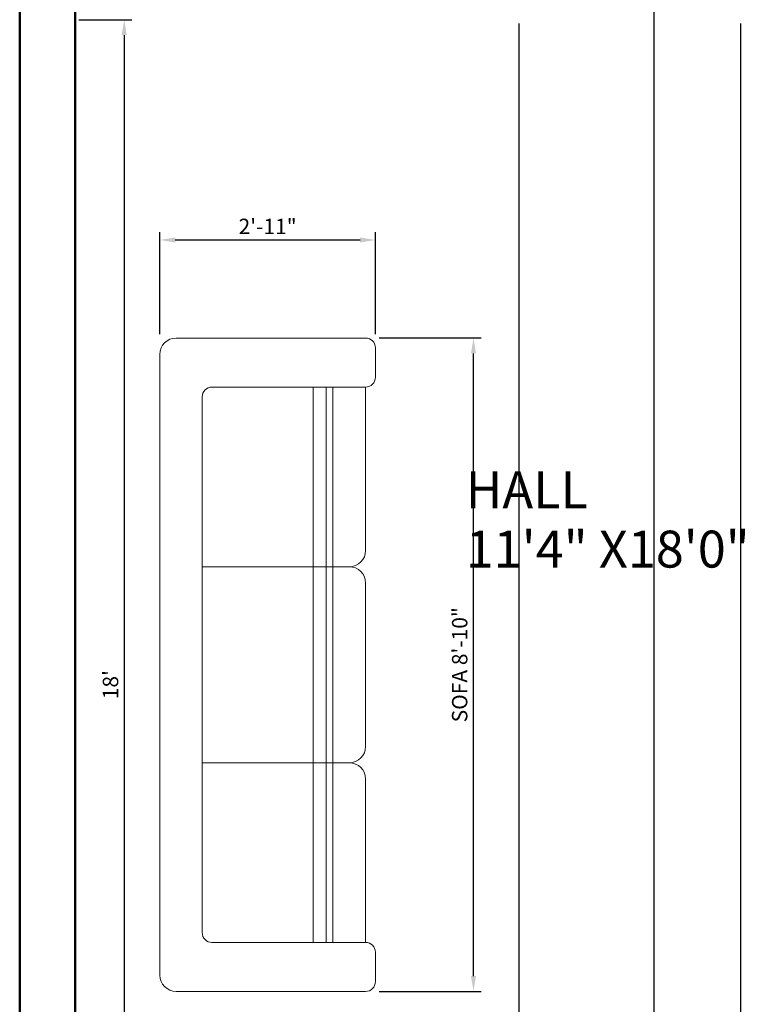
# Model space of a CAD drawing. Units: inches. Extents: x 2385 to 2740, y 1752 to 2305.
# Tile 7 of 15: x 2414 to 2535, y 1981 to 2141. Entities that reach past the tile are written whole.
import ezdxf

# ---------------------------------------------------------------- set-up
doc = ezdxf.new("R2010")
doc.units = ezdxf.units.IN
for name, color, linetype, lineweight in [('A-ANNO-DIMS', 2, 'Continuous', 18), ('A-AREA-IDEN', 7, 'Continuous', 25), ('A-FURN', 9, 'Continuous', 18), ('A-WALL', 7, 'Continuous', 50)]:
    doc.layers.add(name, color=color, linetype=linetype, lineweight=lineweight)
doc.styles.get("Standard").update_dxf_attribs({"font": 'arial.ttf'})
doc.dimstyles.new('Copy of ISO-25', dxfattribs={"dimtxt": 2.5, "dimasz": 2.5, "dimexe": 1.25, "dimexo": 0.625, "dimtad": 1, "dimdec": 1, "dimlunit": 4, "dimtxsty": 'Standard', "dimcen": 2.5, "dimadec": 0, "dimazin": 0, "dimtfac": 1, "dimtdec": 1, "dimtmove": 0, "dimatfit": 3, "dimfxl": 1, "dimarcsym": 0})

# ---------------------------------------------------------------- blocks, each defined once
blk = doc.blocks.new('A$C05BA3A2B')
for p, q in [((0.05, 0.6596), (1.95, 0.6596)), ((0.05, 0.6596), (1.95, 0.6596)), ((0.05, 0.6596), (1.95, 0.6596)), ((0, 0.03), (0, 0.6096)), ((0, 0.03), (0, 0.6096)), ((0, 0.03), (0, 0.6096)), ((2, 0.6096), (2, 0.03)), ((2, 0.6096), (2, 0.03)), ((2, 0.6096), (2, 0.03)), ((1.82, 0.53), (0.18, 0.53)), ((1.82, 0.53), (0.18, 0.53)), ((1.82, 0.53), (0.18, 0.53)), ((0.7, 0.08), (0.7, 0.53)), ((0.7, 0.08), (0.7, 0.53)), ((0.7, 0.08), (0.7, 0.53)), ((1.3, 0.53), (1.3, 0.08)), ((1.3, 0.53), (1.3, 0.08)), ((1.3, 0.53), (1.3, 0.08)), ((0.15, 0.5), (0.15, 0.03)), ((0.15, 0.5), (0.15, 0.03)), ((0.15, 0.5), (0.15, 0.03)), ((1.85, 0.03), (1.85, 0.5)), ((1.85, 0.03), (1.85, 0.5)), ((1.85, 0.03), (1.85, 0.5)), ((1.85, 0.1908), (0.15, 0.1908)), ((1.85, 0.1908), (0.15, 0.1908)), ((1.85, 0.1908), (0.15, 0.1908)), ((1.85, 0.1508), (0.15, 0.1508)), ((1.85, 0.1508), (0.15, 0.1508)), ((1.85, 0.1508), (0.15, 0.1508)), ((1.85, 0.1308), (0.15, 0.1308)), ((1.85, 0.1308), (0.15, 0.1308)), ((1.85, 0.1308), (0.15, 0.1308)), ((0.12, 0), (0.03, 0)), ((0.12, 0), (0.03, 0)), ((0.12, 0), (0.03, 0)), ((0.65, 0.03), (0.15, 0.03)), ((0.65, 0.03), (0.15, 0.03)), ((0.65, 0.03), (0.15, 0.03)), ((1.25, 0.03), (0.75, 0.03)), ((1.25, 0.03), (0.75, 0.03)), ((1.25, 0.03), (0.75, 0.03)), ((1.85, 0.03), (1.35, 0.03)), ((1.85, 0.03), (1.35, 0.03)), ((1.85, 0.03), (1.35, 0.03)), ((1.97, 0), (1.88, 0)), ((1.97, 0), (1.88, 0)), ((1.97, 0), (1.88, 0))]:
    blk.add_line(p, q)
for centre, radius, start, end in [((0.05, 0.6096), 0.05, 90, 180), ((0.05, 0.6096), 0.05, 90, 180), ((0.05, 0.6096), 0.05, 90, 180), ((1.95, 0.6096), 0.05, 0, 90), ((1.95, 0.6096), 0.05, 0, 90), ((1.95, 0.6096), 0.05, 0, 90), ((0.18, 0.5), 0.03, 90, 180), ((0.18, 0.5), 0.03, 90, 180), ((0.18, 0.5), 0.03, 90, 180), ((1.82, 0.5), 0.03, 0, 90), ((1.82, 0.5), 0.03, 0, 90), ((1.82, 0.5), 0.03, 0, 90), ((0.65, 0.08), 0.05, 270, 0), ((0.65, 0.08), 0.05, 270, 0), ((0.65, 0.08), 0.05, 270, 0), ((0.75, 0.08), 0.05, 180, 270), ((0.75, 0.08), 0.05, 180, 270), ((0.75, 0.08), 0.05, 180, 270), ((1.25, 0.08), 0.05, 270, 0), ((1.25, 0.08), 0.05, 270, 0), ((1.25, 0.08), 0.05, 270, 0), ((1.35, 0.08), 0.05, 180, 270), ((1.35, 0.08), 0.05, 180, 270), ((1.35, 0.08), 0.05, 180, 270), ((0.03, 0.03), 0.03, 180, 270), ((0.03, 0.03), 0.03, 180, 270), ((0.03, 0.03), 0.03, 180, 270), ((0.12, 0.03), 0.03, 270, 0), ((0.12, 0.03), 0.03, 270, 0), ((0.12, 0.03), 0.03, 270, 0), ((1.88, 0.03), 0.03, 180, 270), ((1.88, 0.03), 0.03, 180, 270), ((1.88, 0.03), 0.03, 180, 270), ((1.97, 0.03), 0.03, 270, 0), ((1.97, 0.03), 0.03, 270, 0), ((1.97, 0.03), 0.03, 270, 0)]:
    blk.add_arc(centre, radius, start, end)
blk = doc.blocks.new('*D12')
at = {"layer": 'A-ANNO-DIMS', "color": 0, "lineweight": -2, "transparency": 16777216}
for p, q in [((2423.87, 2140.97), (2432.46, 2140.97)), ((2431.21, 2138.47), (2431.21, 1927.47)), ((2423.87, 1924.97), (2432.46, 1924.97))]:
    blk.add_line(p, q, dxfattribs=at)
at = {"layer": 'A-ANNO-DIMS', "color": 0, "transparency": 16777216}
for points in [[(2430.79, 2138.47), (2431.63, 2138.47), (2431.21, 2140.97)], [(2430.79, 1927.47), (2431.63, 1927.47), (2431.21, 1924.97)]]:
    blk.add_solid(points, dxfattribs=at)
at = {"layer": 'Defpoints', "color": 0, "transparency": 16777216}
for p in [(2423.25, 2140.97), (2423.25, 1924.97), (2431.21, 1924.97)]:
    blk.add_point(p, dxfattribs=at)
at = {"layer": 'A-ANNO-DIMS', "color": 0, "transparency": 16777216, "insert": (2429.31, 2032.97), "char_height": 2.5, "attachment_point": 5, "rotation": 90}
blk.add_mtext("18'", dxfattribs=at)
blk = doc.blocks.new('*D30')
at = {"layer": 'A-ANNO-DIMS', "color": 0, "lineweight": -2, "transparency": 16777216}
for p, q in [((2472.61, 2089.28), (2489.16, 2089.28)), ((2487.91, 1985.65), (2487.91, 2086.78)), ((2472.61, 1983.15), (2489.16, 1983.15))]:
    blk.add_line(p, q, dxfattribs=at)
at = {"layer": 'A-ANNO-DIMS', "color": 0, "transparency": 16777216}
for points in [[(2487.49, 2086.78), (2488.32, 2086.78), (2487.91, 2089.28)], [(2487.49, 1985.65), (2488.32, 1985.65), (2487.91, 1983.15)]]:
    blk.add_solid(points, dxfattribs=at)
at = {"layer": 'Defpoints', "color": 0, "transparency": 16777216}
for p in [(2471.99, 2089.28), (2487.91, 2089.28), (2471.99, 1983.15)]:
    blk.add_point(p, dxfattribs=at)
at = {"layer": 'A-ANNO-DIMS', "color": 0, "transparency": 16777216, "insert": (2485.99, 2036.21), "char_height": 2.5, "attachment_point": 5, "rotation": 90}
blk.add_mtext('SOFA 8\'-10"', dxfattribs=at)
blk = doc.blocks.new('*D31')
at = {"layer": 'A-ANNO-DIMS', "color": 0, "lineweight": -2, "transparency": 16777216}
for p, q in [((2436.99, 2089.9), (2436.99, 2106.44)), ((2471.99, 2089.9), (2471.99, 2106.44)), ((2469.49, 2105.19), (2439.49, 2105.19))]:
    blk.add_line(p, q, dxfattribs=at)
at = {"layer": 'A-ANNO-DIMS', "color": 0, "transparency": 16777216}
for points in [[(2439.49, 2105.61), (2439.49, 2104.78), (2436.99, 2105.19)], [(2469.49, 2105.61), (2469.49, 2104.78), (2471.99, 2105.19)]]:
    blk.add_solid(points, dxfattribs=at)
at = {"layer": 'Defpoints', "color": 0, "transparency": 16777216}
for p in [(2436.99, 2105.19), (2436.99, 2089.28), (2471.99, 2089.28)]:
    blk.add_point(p, dxfattribs=at)
at = {"layer": 'A-ANNO-DIMS', "color": 0, "transparency": 16777216, "insert": (2454.49, 2107.07), "char_height": 2.5, "attachment_point": 5}
blk.add_mtext('2\'-11"', dxfattribs=at)
blk = doc.blocks.new('*D37')
at = {"layer": 'A-ANNO-DIMS', "color": 0, "lineweight": -2, "transparency": 16777216}
for p, q in [((2495.25, 2140.34), (2495.25, 1752.1)), ((2531.25, 2140.34), (2531.25, 1752.1)), ((2497.75, 1753.35), (2528.75, 1753.35))]:
    blk.add_line(p, q, dxfattribs=at)
at = {"layer": 'A-ANNO-DIMS', "color": 0, "transparency": 16777216}
for points in [[(2497.75, 1753.77), (2497.75, 1752.94), (2495.25, 1753.35)], [(2528.75, 1753.77), (2528.75, 1752.94), (2531.25, 1753.35)]]:
    blk.add_solid(points, dxfattribs=at)
at = {"layer": 'Defpoints', "color": 0, "transparency": 16777216}
for p in [(2495.25, 2140.97), (2531.25, 2140.97), (2531.25, 1753.35)]:
    blk.add_point(p, dxfattribs=at)
at = {"layer": 'A-ANNO-DIMS', "color": 0, "transparency": 16777216, "insert": (2513.25, 1755.25), "char_height": 2.5, "attachment_point": 5}
blk.add_mtext('3\'-0"', dxfattribs=at)
blk = doc.blocks.new('*D48')
at = {"layer": 'A-ANNO-DIMS', "color": 0, "lineweight": -2, "transparency": 16777216}
for p, q in [((2517.25, 1916.59), (2517.25, 2302.84)), ((2553.25, 1916.59), (2553.25, 2302.84)), ((2519.75, 2301.59), (2550.75, 2301.59))]:
    blk.add_line(p, q, dxfattribs=at)
at = {"layer": 'A-ANNO-DIMS', "color": 0, "transparency": 16777216}
for points in [[(2519.75, 2302), (2519.75, 2301.17), (2517.25, 2301.59)], [(2550.75, 2302), (2550.75, 2301.17), (2553.25, 2301.59)]]:
    blk.add_solid(points, dxfattribs=at)
at = {"layer": 'Defpoints', "color": 0, "transparency": 16777216}
for p in [(2553.25, 2301.59), (2517.25, 1915.97), (2553.25, 1915.97)]:
    blk.add_point(p, dxfattribs=at)
at = {"layer": 'A-ANNO-DIMS', "color": 0, "transparency": 16777216, "insert": (2535.25, 2303.49), "char_height": 2.5, "attachment_point": 5}
blk.add_mtext('3\'-0"', dxfattribs=at)

msp = doc.modelspace()

# ---------------------------------------------------------------- linework, layer by layer
at = {"layer": 'A-WALL'}
for p, q in [((2414.25, 1924.97), (2414.25, 2266.97)), ((2423.25, 2146.97), (2423.25, 2140.97)), ((2423.25, 2140.97), (2423.25, 1924.97)), ((2423.25, 2140.97), (2423.25, 1924.97))]:
    msp.add_line(p, q, dxfattribs=at)

# ---------------------------------------------------------------- block references
at = {"layer": 'A-FURN', "xscale": 53.0614237901251, "yscale": 53.0614237901251, "zscale": 53.0614237901251, "rotation": 90}
msp.add_blockref('A$C05BA3A2B', (2471.99, 1983.15), dxfattribs=at)

# ---------------------------------------------------------------- texts
at = {"layer": 'A-AREA-IDEN'}
for s, p in [('HALL', (2486.65, 2061.63)), ('11\'4" X18\'0"', (2486.65, 2051.99))]:
    msp.add_text(s, height=6, dxfattribs=at).set_placement(p)

# ---------------------------------------------------------------- dimensions: what is measured, and where the dimension line sits
at = {"layer": 'A-ANNO-DIMS'}
for base, p1, p2, picture, middle in [((2553.25, 2301.59), (2517.25, 1915.97), (2553.25, 1915.97), '*D48', (2535.25, 2303.49)), ((2531.25, 1753.35), (2495.25, 2140.97), (2531.25, 2140.97), '*D37', (2513.25, 1755.25))]:
    dim = msp.add_linear_dim(base=base, p1=p1, p2=p2, dimstyle='Copy of ISO-25', override={"dimdec": 1, "dimlfac": 1, "dimrnd": 0, "dimzin": 1, "dimdsep": 46, "dimlunit": 4, "dimfrac": 2}, dxfattribs=at)
    dim.commit()
    dim.dimension.update_dxf_attribs({"geometry": picture, "text_midpoint": middle})
for base, p1, p2, angle, override, picture, middle in [((2431.21, 1924.97), (2423.25, 2140.97), (2423.25, 1924.97), 90, {"dimclrd": 0, "dimclre": 0, "dimclrt": 0}, '*D12', (2429.31, 2032.97)), ((2436.99, 2105.19), (2471.99, 2089.28), (2436.99, 2089.28), 180, {"dimdec": 1, "dimlfac": 1, "dimrnd": 0, "dimzin": 1, "dimdsep": 46, "dimlunit": 4, "dimfrac": 2}, '*D31', (2454.49, 2107.07))]:
    dim = msp.add_linear_dim(base=base, p1=p1, p2=p2, angle=angle, dimstyle='Copy of ISO-25', override=override, dxfattribs=at)
    dim.commit()
    dim.dimension.update_dxf_attribs({"geometry": picture, "text_midpoint": middle})
dim = msp.add_linear_dim(base=(2487.91, 2089.28), p1=(2471.99, 1983.15), p2=(2471.99, 2089.28), angle=90, text='SOFA <>', dimstyle='Copy of ISO-25', override={"dimdec": 1, "dimlfac": 1, "dimrnd": 0, "dimzin": 1, "dimdsep": 46, "dimlunit": 4, "dimfrac": 2}, dxfattribs=at)
dim.commit()
dim.dimension.update_dxf_attribs({"geometry": '*D30', "text_midpoint": (2485.99, 2036.21)})

doc.saveas('drawing.dxf')
